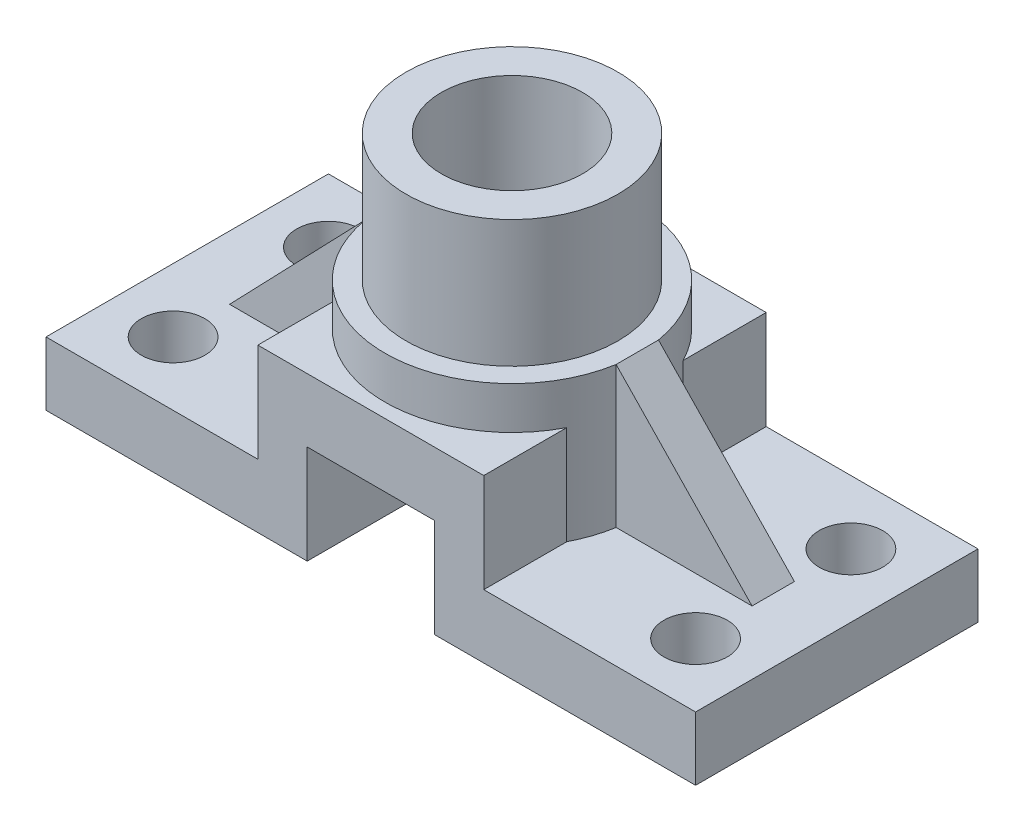
ISO-10303-21;
HEADER;
FILE_DESCRIPTION(('STEP AP214'),'2;1');
FILE_NAME('part.step','',(''),(''),'','','');
FILE_SCHEMA(('AUTOMOTIVE_DESIGN { 1 0 10303 214 1 1 1 1 }'));
ENDSEC;
DATA;
#1=APPLICATION_CONTEXT('core data for automotive mechanical design processes');
#2=APPLICATION_PROTOCOL_DEFINITION('international standard','automotive_design',2000,#1);
#3=PRODUCT_CONTEXT('',#1,'mechanical');
#4=PRODUCT('Part','Part','',(#3));
#5=PRODUCT_RELATED_PRODUCT_CATEGORY('part','',(#4));
#6=PRODUCT_DEFINITION_FORMATION('','',#4);
#7=PRODUCT_DEFINITION_CONTEXT('part definition',#1,'design');
#8=PRODUCT_DEFINITION('design','',#6,#7);
#9=PRODUCT_DEFINITION_SHAPE('','',#8);
#10=(LENGTH_UNIT() NAMED_UNIT(*) SI_UNIT(.MILLI.,.METRE.));
#11=(NAMED_UNIT(*) PLANE_ANGLE_UNIT() SI_UNIT($,.RADIAN.));
#12=(NAMED_UNIT(*) SI_UNIT($,.STERADIAN.) SOLID_ANGLE_UNIT());
#13=UNCERTAINTY_MEASURE_WITH_UNIT(LENGTH_MEASURE(1.E-05),#10,'distance_accuracy_value','');
#14=(GEOMETRIC_REPRESENTATION_CONTEXT(3) GLOBAL_UNCERTAINTY_ASSIGNED_CONTEXT((#13)) GLOBAL_UNIT_ASSIGNED_CONTEXT((#10,
#11,#12)) REPRESENTATION_CONTEXT('',''));
#15=CARTESIAN_POINT('',(0.,0.,0.));
#16=DIRECTION('',(0.,0.,1.));
#17=DIRECTION('',(1.,0.,0.));
#18=AXIS2_PLACEMENT_3D('',#15,#16,#17);
#19=CARTESIAN_POINT('',(-16.,9.,20.));
#20=DIRECTION('',(0.,-1.,0.));
#21=DIRECTION('',(1.,0.,0.));
#22=AXIS2_PLACEMENT_3D('',#19,#20,#21);
#23=PLANE('',#22);
#24=CARTESIAN_POINT('',(-37.,9.,-11.));
#25=DIRECTION('',(0.,-1.,0.));
#26=DIRECTION('',(1.,0.,0.));
#27=AXIS2_PLACEMENT_3D('',#24,#25,#26);
#28=CIRCLE('',#27,4.5);
#29=CARTESIAN_POINT('',(-32.5,9.,-11.));
#30=VERTEX_POINT('',#29);
#31=EDGE_CURVE('E214',#30,#30,#28,.T.);
#32=ORIENTED_EDGE('',*,*,#31,.T.);
#33=EDGE_LOOP('',(#32));
#34=FACE_BOUND('',#33,.T.);
#35=DIRECTION('',(0.,0.,-1.));
#36=VECTOR('',#35,1.);
#37=CARTESIAN_POINT('',(-37.,9.00000000000001,-3.));
#38=LINE('',#37,#36);
#39=CARTESIAN_POINT('',(-37.,9.00000000000001,3.00000000000001));
#40=VERTEX_POINT('',#39);
#41=CARTESIAN_POINT('',(-37.,9.00000000000001,-3.));
#42=VERTEX_POINT('',#41);
#43=EDGE_CURVE('E187',#40,#42,#38,.T.);
#44=ORIENTED_EDGE('',*,*,#43,.T.);
#45=DIRECTION('',(1.,0.,0.));
#46=VECTOR('',#45,1.);
#47=CARTESIAN_POINT('',(-37.,9.00000000000001,-3.));
#48=LINE('',#47,#46);
#49=CARTESIAN_POINT('',(-17.7482393492988,9.00000000000001,-3.));
#50=VERTEX_POINT('',#49);
#51=EDGE_CURVE('E199',#42,#50,#48,.T.);
#52=ORIENTED_EDGE('',*,*,#51,.T.);
#53=CARTESIAN_POINT('',(0.,9.00000000000001,0.));
#54=DIRECTION('',(0.,-1.,0.));
#55=DIRECTION('',(1.,0.,0.));
#56=AXIS2_PLACEMENT_3D('',#53,#54,#55);
#57=CIRCLE('',#56,18.);
#58=CARTESIAN_POINT('',(-16.,9.,-8.24621125123532));
#59=VERTEX_POINT('',#58);
#60=EDGE_CURVE('E276',#59,#50,#57,.F.);
#61=ORIENTED_EDGE('',*,*,#60,.F.);
#62=DIRECTION('',(0.,0.,-1.));
#63=VECTOR('',#62,1.);
#64=CARTESIAN_POINT('',(-16.,9.,20.));
#65=LINE('',#64,#63);
#66=CARTESIAN_POINT('',(-16.,9.,-20.));
#67=VERTEX_POINT('',#66);
#68=EDGE_CURVE('E359',#59,#67,#65,.T.);
#69=ORIENTED_EDGE('',*,*,#68,.T.);
#70=DIRECTION('',(-1.,0.,0.));
#71=VECTOR('',#70,1.);
#72=CARTESIAN_POINT('',(-16.,9.,-20.));
#73=LINE('',#72,#71);
#74=CARTESIAN_POINT('',(-46.,9.,-20.));
#75=VERTEX_POINT('',#74);
#76=EDGE_CURVE('E307',#67,#75,#73,.T.);
#77=ORIENTED_EDGE('',*,*,#76,.T.);
#78=DIRECTION('',(0.,0.,-1.));
#79=VECTOR('',#78,1.);
#80=CARTESIAN_POINT('',(-46.,9.,20.));
#81=LINE('',#80,#79);
#82=CARTESIAN_POINT('',(-46.,9.,20.));
#83=VERTEX_POINT('',#82);
#84=EDGE_CURVE('E328',#83,#75,#81,.T.);
#85=ORIENTED_EDGE('',*,*,#84,.F.);
#86=DIRECTION('',(-1.,0.,0.));
#87=VECTOR('',#86,1.);
#88=CARTESIAN_POINT('',(-16.,9.,20.));
#89=LINE('',#88,#87);
#90=CARTESIAN_POINT('',(-16.,9.,20.));
#91=VERTEX_POINT('',#90);
#92=EDGE_CURVE('E330',#91,#83,#89,.T.);
#93=ORIENTED_EDGE('',*,*,#92,.F.);
#94=CARTESIAN_POINT('',(-16.,9.00000000000001,8.24621125123532));
#95=VERTEX_POINT('',#94);
#96=EDGE_CURVE('E356',#91,#95,#65,.T.);
#97=ORIENTED_EDGE('',*,*,#96,.T.);
#98=CARTESIAN_POINT('',(-17.7482393492988,9.00000000000001,3.));
#99=VERTEX_POINT('',#98);
#100=EDGE_CURVE('E212',#99,#95,#57,.F.);
#101=ORIENTED_EDGE('',*,*,#100,.F.);
#102=DIRECTION('',(-1.,0.,0.));
#103=VECTOR('',#102,1.);
#104=CARTESIAN_POINT('',(-37.,9.00000000000001,3.));
#105=LINE('',#104,#103);
#106=EDGE_CURVE('E206',#99,#40,#105,.T.);
#107=ORIENTED_EDGE('',*,*,#106,.T.);
#108=EDGE_LOOP('',(#44,#52,#61,#69,#77,#85,#93,#97,#101,#107));
#109=FACE_BOUND('',#108,.T.);
#110=CARTESIAN_POINT('',(-37.,9.,11.));
#111=DIRECTION('',(0.,-1.,0.));
#112=DIRECTION('',(1.,0.,0.));
#113=AXIS2_PLACEMENT_3D('',#110,#111,#112);
#114=CIRCLE('',#113,4.5);
#115=CARTESIAN_POINT('',(-32.5,9.,11.));
#116=VERTEX_POINT('',#115);
#117=EDGE_CURVE('E235',#116,#116,#114,.T.);
#118=ORIENTED_EDGE('',*,*,#117,.T.);
#119=EDGE_LOOP('',(#118));
#120=FACE_BOUND('',#119,.T.);
#121=ADVANCED_FACE('F39',(#34,#109,#120),#23,.F.);
#122=CARTESIAN_POINT('',(0.,29.,0.));
#123=DIRECTION('',(0.,-1.,0.));
#124=DIRECTION('',(1.,0.,0.));
#125=AXIS2_PLACEMENT_3D('',#122,#123,#124);
#126=CYLINDRICAL_SURFACE('',#125,18.);
#127=DIRECTION('',(0.,1.,0.));
#128=VECTOR('',#127,1.);
#129=CARTESIAN_POINT('',(-17.7482393492988,-11.1650759520485,-3.));
#130=LINE('',#129,#128);
#131=CARTESIAN_POINT('',(-17.7482393492988,29.,-3.));
#132=VERTEX_POINT('',#131);
#133=EDGE_CURVE('E221',#50,#132,#130,.T.);
#134=ORIENTED_EDGE('',*,*,#133,.T.);
#135=CARTESIAN_POINT('',(0.,29.,0.));
#136=DIRECTION('',(0.,1.,0.));
#137=DIRECTION('',(-1.,0.,0.));
#138=AXIS2_PLACEMENT_3D('',#135,#136,#137);
#139=CIRCLE('',#138,18.);
#140=CARTESIAN_POINT('',(17.7482393492988,29.,-3.));
#141=VERTEX_POINT('',#140);
#142=EDGE_CURVE('E278',#141,#132,#139,.T.);
#143=ORIENTED_EDGE('',*,*,#142,.F.);
#144=DIRECTION('',(0.,1.,0.));
#145=VECTOR('',#144,1.);
#146=CARTESIAN_POINT('',(17.7482393492988,-11.1650759520485,-3.));
#147=LINE('',#146,#145);
#148=CARTESIAN_POINT('',(17.7482393492988,9.,-3.));
#149=VERTEX_POINT('',#148);
#150=EDGE_CURVE('E241',#149,#141,#147,.T.);
#151=ORIENTED_EDGE('',*,*,#150,.F.);
#152=CARTESIAN_POINT('',(0.,9.00000000000001,0.));
#153=DIRECTION('',(0.,1.,0.));
#154=DIRECTION('',(-1.,0.,0.));
#155=AXIS2_PLACEMENT_3D('',#152,#153,#154);
#156=CIRCLE('',#155,18.);
#157=CARTESIAN_POINT('',(16.,9.,-8.24621125123532));
#158=VERTEX_POINT('',#157);
#159=EDGE_CURVE('E63',#149,#158,#156,.T.);
#160=ORIENTED_EDGE('',*,*,#159,.T.);
#161=DIRECTION('',(0.,-1.,0.));
#162=VECTOR('',#161,1.);
#163=CARTESIAN_POINT('',(16.,29.,-8.24621125123533));
#164=LINE('',#163,#162);
#165=CARTESIAN_POINT('',(16.,23.,-8.24621125123533));
#166=VERTEX_POINT('',#165);
#167=EDGE_CURVE('E291',#158,#166,#164,.F.);
#168=ORIENTED_EDGE('',*,*,#167,.T.);
#169=CARTESIAN_POINT('',(0.,23.,0.));
#170=DIRECTION('',(0.,-1.,0.));
#171=DIRECTION('',(0.,0.,-1.));
#172=AXIS2_PLACEMENT_3D('',#169,#170,#171);
#173=CIRCLE('',#172,18.);
#174=CARTESIAN_POINT('',(-16.,23.,-8.24621125123531));
#175=VERTEX_POINT('',#174);
#176=EDGE_CURVE('E286',#166,#175,#173,.F.);
#177=ORIENTED_EDGE('',*,*,#176,.T.);
#178=DIRECTION('',(0.,-1.,0.));
#179=VECTOR('',#178,1.);
#180=CARTESIAN_POINT('',(-16.,29.,-8.24621125123531));
#181=LINE('',#180,#179);
#182=EDGE_CURVE('E281',#175,#59,#181,.T.);
#183=ORIENTED_EDGE('',*,*,#182,.T.);
#184=ORIENTED_EDGE('',*,*,#60,.T.);
#185=EDGE_LOOP('',(#134,#143,#151,#160,#168,#177,#183,#184));
#186=FACE_BOUND('',#185,.T.);
#187=ADVANCED_FACE('F420',(#186),#126,.T.);
#188=DIRECTION('',(0.,1.,0.));
#189=VECTOR('',#188,1.);
#190=CARTESIAN_POINT('',(-17.7482393492988,-11.1650759520485,3.));
#191=LINE('',#190,#189);
#192=CARTESIAN_POINT('',(-17.7482393492988,29.,3.00000000000001));
#193=VERTEX_POINT('',#192);
#194=EDGE_CURVE('E203',#99,#193,#191,.T.);
#195=ORIENTED_EDGE('',*,*,#194,.F.);
#196=ORIENTED_EDGE('',*,*,#100,.T.);
#197=DIRECTION('',(0.,-1.,0.));
#198=VECTOR('',#197,1.);
#199=CARTESIAN_POINT('',(-16.,29.,8.24621125123531));
#200=LINE('',#199,#198);
#201=CARTESIAN_POINT('',(-16.,23.,8.24621125123531));
#202=VERTEX_POINT('',#201);
#203=EDGE_CURVE('E298',#95,#202,#200,.F.);
#204=ORIENTED_EDGE('',*,*,#203,.T.);
#205=CARTESIAN_POINT('',(16.,23.,8.24621125123533));
#206=VERTEX_POINT('',#205);
#207=EDGE_CURVE('E294',#202,#206,#173,.F.);
#208=ORIENTED_EDGE('',*,*,#207,.T.);
#209=DIRECTION('',(0.,-1.,0.));
#210=VECTOR('',#209,1.);
#211=CARTESIAN_POINT('',(16.,29.,8.24621125123533));
#212=LINE('',#211,#210);
#213=CARTESIAN_POINT('',(16.,9.,8.24621125123532));
#214=VERTEX_POINT('',#213);
#215=EDGE_CURVE('E297',#206,#214,#212,.T.);
#216=ORIENTED_EDGE('',*,*,#215,.T.);
#217=CARTESIAN_POINT('',(17.7482393492988,9.00000000000001,3.));
#218=VERTEX_POINT('',#217);
#219=EDGE_CURVE('E284',#214,#218,#156,.T.);
#220=ORIENTED_EDGE('',*,*,#219,.T.);
#221=DIRECTION('',(0.,1.,0.));
#222=VECTOR('',#221,1.);
#223=CARTESIAN_POINT('',(17.7482393492988,-11.1650759520485,3.));
#224=LINE('',#223,#222);
#225=CARTESIAN_POINT('',(17.7482393492988,29.,3.00000000000001));
#226=VERTEX_POINT('',#225);
#227=EDGE_CURVE('E243',#218,#226,#224,.T.);
#228=ORIENTED_EDGE('',*,*,#227,.T.);
#229=EDGE_CURVE('E282',#193,#226,#139,.T.);
#230=ORIENTED_EDGE('',*,*,#229,.F.);
#231=EDGE_LOOP('',(#195,#196,#204,#208,#216,#220,#228,#230));
#232=FACE_BOUND('',#231,.T.);
#233=ADVANCED_FACE('F426',(#232),#126,.T.);
#234=CARTESIAN_POINT('',(-9.,0.,20.));
#235=DIRECTION('',(-1.,0.,0.));
#236=DIRECTION('',(0.,0.,1.));
#237=AXIS2_PLACEMENT_3D('',#234,#235,#236);
#238=PLANE('',#237);
#239=DIRECTION('',(0.,0.,-1.));
#240=VECTOR('',#239,1.);
#241=CARTESIAN_POINT('',(-9.,14.,20.));
#242=LINE('',#241,#240);
#243=CARTESIAN_POINT('',(-9.,14.,20.));
#244=VERTEX_POINT('',#243);
#245=CARTESIAN_POINT('',(-9.,14.,-20.));
#246=VERTEX_POINT('',#245);
#247=EDGE_CURVE('E384',#244,#246,#242,.T.);
#248=ORIENTED_EDGE('',*,*,#247,.F.);
#249=DIRECTION('',(0.,1.,0.));
#250=VECTOR('',#249,1.);
#251=CARTESIAN_POINT('',(-9.,0.,20.));
#252=LINE('',#251,#250);
#253=CARTESIAN_POINT('',(-9.,0.,20.));
#254=VERTEX_POINT('',#253);
#255=EDGE_CURVE('E310',#254,#244,#252,.T.);
#256=ORIENTED_EDGE('',*,*,#255,.F.);
#257=DIRECTION('',(0.,0.,-1.));
#258=VECTOR('',#257,1.);
#259=CARTESIAN_POINT('',(-9.,0.,20.));
#260=LINE('',#259,#258);
#261=CARTESIAN_POINT('',(-9.,0.,-20.));
#262=VERTEX_POINT('',#261);
#263=EDGE_CURVE('E389',#254,#262,#260,.T.);
#264=ORIENTED_EDGE('',*,*,#263,.T.);
#265=DIRECTION('',(0.,1.,0.));
#266=VECTOR('',#265,1.);
#267=CARTESIAN_POINT('',(-9.,0.,-20.));
#268=LINE('',#267,#266);
#269=EDGE_CURVE('E331',#262,#246,#268,.T.);
#270=ORIENTED_EDGE('',*,*,#269,.T.);
#271=EDGE_LOOP('',(#248,#256,#264,#270));
#272=FACE_BOUND('',#271,.T.);
#273=ADVANCED_FACE('F465',(#272),#238,.F.);
#274=CARTESIAN_POINT('',(9.,14.,20.));
#275=DIRECTION('',(1.,0.,0.));
#276=DIRECTION('',(0.,0.,-1.));
#277=AXIS2_PLACEMENT_3D('',#274,#275,#276);
#278=PLANE('',#277);
#279=DIRECTION('',(0.,-1.,0.));
#280=VECTOR('',#279,1.);
#281=CARTESIAN_POINT('',(9.,14.,-20.));
#282=LINE('',#281,#280);
#283=CARTESIAN_POINT('',(9.,14.,-20.));
#284=VERTEX_POINT('',#283);
#285=CARTESIAN_POINT('',(9.,0.,-20.));
#286=VERTEX_POINT('',#285);
#287=EDGE_CURVE('E337',#284,#286,#282,.T.);
#288=ORIENTED_EDGE('',*,*,#287,.T.);
#289=DIRECTION('',(0.,0.,-1.));
#290=VECTOR('',#289,1.);
#291=CARTESIAN_POINT('',(9.,0.,20.));
#292=LINE('',#291,#290);
#293=CARTESIAN_POINT('',(9.,0.,20.));
#294=VERTEX_POINT('',#293);
#295=EDGE_CURVE('E379',#294,#286,#292,.T.);
#296=ORIENTED_EDGE('',*,*,#295,.F.);
#297=DIRECTION('',(0.,-1.,0.));
#298=VECTOR('',#297,1.);
#299=CARTESIAN_POINT('',(9.,14.,20.));
#300=LINE('',#299,#298);
#301=CARTESIAN_POINT('',(9.,14.,20.));
#302=VERTEX_POINT('',#301);
#303=EDGE_CURVE('E311',#302,#294,#300,.T.);
#304=ORIENTED_EDGE('',*,*,#303,.F.);
#305=DIRECTION('',(0.,0.,-1.));
#306=VECTOR('',#305,1.);
#307=CARTESIAN_POINT('',(9.,14.,20.));
#308=LINE('',#307,#306);
#309=EDGE_CURVE('E382',#302,#284,#308,.T.);
#310=ORIENTED_EDGE('',*,*,#309,.T.);
#311=EDGE_LOOP('',(#288,#296,#304,#310));
#312=FACE_BOUND('',#311,.T.);
#313=ADVANCED_FACE('F446',(#312),#278,.F.);
#314=CARTESIAN_POINT('',(16.,9.,20.));
#315=DIRECTION('',(-1.,0.,0.));
#316=DIRECTION('',(0.,0.,1.));
#317=AXIS2_PLACEMENT_3D('',#314,#315,#316);
#318=PLANE('',#317);
#319=ORIENTED_EDGE('',*,*,#167,.F.);
#320=DIRECTION('',(0.,0.,-1.));
#321=VECTOR('',#320,1.);
#322=CARTESIAN_POINT('',(16.,9.,20.));
#323=LINE('',#322,#321);
#324=CARTESIAN_POINT('',(16.,9.,-20.));
#325=VERTEX_POINT('',#324);
#326=EDGE_CURVE('E367',#158,#325,#323,.T.);
#327=ORIENTED_EDGE('',*,*,#326,.T.);
#328=DIRECTION('',(0.,1.,0.));
#329=VECTOR('',#328,1.);
#330=CARTESIAN_POINT('',(16.,9.,-20.));
#331=LINE('',#330,#329);
#332=CARTESIAN_POINT('',(16.,23.,-20.));
#333=VERTEX_POINT('',#332);
#334=EDGE_CURVE('E350',#325,#333,#331,.T.);
#335=ORIENTED_EDGE('',*,*,#334,.T.);
#336=DIRECTION('',(0.,0.,-1.));
#337=VECTOR('',#336,1.);
#338=CARTESIAN_POINT('',(16.,23.,20.));
#339=LINE('',#338,#337);
#340=EDGE_CURVE('E368',#166,#333,#339,.T.);
#341=ORIENTED_EDGE('',*,*,#340,.F.);
#342=EDGE_LOOP('',(#319,#327,#335,#341));
#343=FACE_BOUND('',#342,.T.);
#344=ADVANCED_FACE('F441',(#343),#318,.F.);
#345=ORIENTED_EDGE('',*,*,#215,.F.);
#346=CARTESIAN_POINT('',(16.,23.,20.));
#347=VERTEX_POINT('',#346);
#348=EDGE_CURVE('E370',#347,#206,#339,.T.);
#349=ORIENTED_EDGE('',*,*,#348,.F.);
#350=DIRECTION('',(0.,1.,0.));
#351=VECTOR('',#350,1.);
#352=CARTESIAN_POINT('',(16.,9.,20.));
#353=LINE('',#352,#351);
#354=CARTESIAN_POINT('',(16.,9.,20.));
#355=VERTEX_POINT('',#354);
#356=EDGE_CURVE('E321',#355,#347,#353,.T.);
#357=ORIENTED_EDGE('',*,*,#356,.F.);
#358=EDGE_CURVE('E371',#355,#214,#323,.T.);
#359=ORIENTED_EDGE('',*,*,#358,.T.);
#360=EDGE_LOOP('',(#345,#349,#357,#359));
#361=FACE_BOUND('',#360,.T.);
#362=ADVANCED_FACE('F450',(#361),#318,.F.);
#363=CARTESIAN_POINT('',(16.,23.,20.));
#364=DIRECTION('',(0.,-1.,0.));
#365=DIRECTION('',(0.,0.,-1.));
#366=AXIS2_PLACEMENT_3D('',#363,#364,#365);
#367=PLANE('',#366);
#368=ORIENTED_EDGE('',*,*,#207,.F.);
#369=DIRECTION('',(0.,0.,-1.));
#370=VECTOR('',#369,1.);
#371=CARTESIAN_POINT('',(-16.,23.,20.));
#372=LINE('',#371,#370);
#373=CARTESIAN_POINT('',(-16.,23.,20.));
#374=VERTEX_POINT('',#373);
#375=EDGE_CURVE('E361',#374,#202,#372,.T.);
#376=ORIENTED_EDGE('',*,*,#375,.F.);
#377=DIRECTION('',(-1.,0.,0.));
#378=VECTOR('',#377,1.);
#379=CARTESIAN_POINT('',(16.,23.,20.));
#380=LINE('',#379,#378);
#381=EDGE_CURVE('E323',#347,#374,#380,.T.);
#382=ORIENTED_EDGE('',*,*,#381,.F.);
#383=ORIENTED_EDGE('',*,*,#348,.T.);
#384=EDGE_LOOP('',(#368,#376,#382,#383));
#385=FACE_BOUND('',#384,.T.);
#386=ADVANCED_FACE('F436',(#385),#367,.F.);
#387=CARTESIAN_POINT('',(-16.,23.,20.));
#388=DIRECTION('',(1.,0.,0.));
#389=DIRECTION('',(0.,0.,-1.));
#390=AXIS2_PLACEMENT_3D('',#387,#388,#389);
#391=PLANE('',#390);
#392=ORIENTED_EDGE('',*,*,#203,.F.);
#393=ORIENTED_EDGE('',*,*,#96,.F.);
#394=DIRECTION('',(0.,-1.,0.));
#395=VECTOR('',#394,1.);
#396=CARTESIAN_POINT('',(-16.,23.,20.));
#397=LINE('',#396,#395);
#398=EDGE_CURVE('E324',#374,#91,#397,.T.);
#399=ORIENTED_EDGE('',*,*,#398,.F.);
#400=ORIENTED_EDGE('',*,*,#375,.T.);
#401=EDGE_LOOP('',(#392,#393,#399,#400));
#402=FACE_BOUND('',#401,.T.);
#403=ADVANCED_FACE('F435',(#402),#391,.F.);
#404=ORIENTED_EDGE('',*,*,#182,.F.);
#405=CARTESIAN_POINT('',(-16.,23.,-20.));
#406=VERTEX_POINT('',#405);
#407=EDGE_CURVE('E362',#175,#406,#372,.T.);
#408=ORIENTED_EDGE('',*,*,#407,.T.);
#409=DIRECTION('',(0.,-1.,0.));
#410=VECTOR('',#409,1.);
#411=CARTESIAN_POINT('',(-16.,23.,-20.));
#412=LINE('',#411,#410);
#413=EDGE_CURVE('E351',#406,#67,#412,.T.);
#414=ORIENTED_EDGE('',*,*,#413,.T.);
#415=ORIENTED_EDGE('',*,*,#68,.F.);
#416=EDGE_LOOP('',(#404,#408,#414,#415));
#417=FACE_BOUND('',#416,.T.);
#418=ADVANCED_FACE('F434',(#417),#391,.F.);
#419=CARTESIAN_POINT('',(-46.,9.,20.));
#420=DIRECTION('',(1.,0.,0.));
#421=DIRECTION('',(0.,0.,-1.));
#422=AXIS2_PLACEMENT_3D('',#419,#420,#421);
#423=PLANE('',#422);
#424=DIRECTION('',(0.,-1.,0.));
#425=VECTOR('',#424,1.);
#426=CARTESIAN_POINT('',(-46.,9.,-20.));
#427=LINE('',#426,#425);
#428=CARTESIAN_POINT('',(-46.,0.,-20.));
#429=VERTEX_POINT('',#428);
#430=EDGE_CURVE('E305',#75,#429,#427,.T.);
#431=ORIENTED_EDGE('',*,*,#430,.T.);
#432=DIRECTION('',(0.,0.,-1.));
#433=VECTOR('',#432,1.);
#434=CARTESIAN_POINT('',(-46.,0.,20.));
#435=LINE('',#434,#433);
#436=CARTESIAN_POINT('',(-46.,0.,20.));
#437=VERTEX_POINT('',#436);
#438=EDGE_CURVE('E393',#437,#429,#435,.T.);
#439=ORIENTED_EDGE('',*,*,#438,.F.);
#440=DIRECTION('',(0.,-1.,0.));
#441=VECTOR('',#440,1.);
#442=CARTESIAN_POINT('',(-46.,9.,20.));
#443=LINE('',#442,#441);
#444=EDGE_CURVE('E303',#83,#437,#443,.T.);
#445=ORIENTED_EDGE('',*,*,#444,.F.);
#446=ORIENTED_EDGE('',*,*,#84,.T.);
#447=EDGE_LOOP('',(#431,#439,#445,#446));
#448=FACE_BOUND('',#447,.T.);
#449=ADVANCED_FACE('F41',(#448),#423,.F.);
#450=CARTESIAN_POINT('',(-46.,0.,20.));
#451=DIRECTION('',(0.,1.,0.));
#452=DIRECTION('',(0.,0.,1.));
#453=AXIS2_PLACEMENT_3D('',#450,#451,#452);
#454=PLANE('',#453);
#455=CARTESIAN_POINT('',(-37.,0.,11.));
#456=DIRECTION('',(0.,-1.,0.));
#457=DIRECTION('',(1.,0.,0.));
#458=AXIS2_PLACEMENT_3D('',#455,#456,#457);
#459=CIRCLE('',#458,4.5);
#460=CARTESIAN_POINT('',(-32.5,0.,11.));
#461=VERTEX_POINT('',#460);
#462=EDGE_CURVE('E226',#461,#461,#459,.T.);
#463=ORIENTED_EDGE('',*,*,#462,.F.);
#464=EDGE_LOOP('',(#463));
#465=FACE_BOUND('',#464,.T.);
#466=CARTESIAN_POINT('',(-37.,0.,-11.));
#467=DIRECTION('',(0.,-1.,0.));
#468=DIRECTION('',(1.,0.,0.));
#469=AXIS2_PLACEMENT_3D('',#466,#467,#468);
#470=CIRCLE('',#469,4.5);
#471=CARTESIAN_POINT('',(-32.5,0.,-11.));
#472=VERTEX_POINT('',#471);
#473=EDGE_CURVE('E217',#472,#472,#470,.T.);
#474=ORIENTED_EDGE('',*,*,#473,.F.);
#475=EDGE_LOOP('',(#474));
#476=FACE_BOUND('',#475,.T.);
#477=DIRECTION('',(1.,0.,0.));
#478=VECTOR('',#477,1.);
#479=CARTESIAN_POINT('',(-46.,0.,-20.));
#480=LINE('',#479,#478);
#481=EDGE_CURVE('E335',#429,#262,#480,.T.);
#482=ORIENTED_EDGE('',*,*,#481,.T.);
#483=ORIENTED_EDGE('',*,*,#263,.F.);
#484=DIRECTION('',(1.,0.,0.));
#485=VECTOR('',#484,1.);
#486=CARTESIAN_POINT('',(-46.,0.,20.));
#487=LINE('',#486,#485);
#488=EDGE_CURVE('E308',#437,#254,#487,.T.);
#489=ORIENTED_EDGE('',*,*,#488,.F.);
#490=ORIENTED_EDGE('',*,*,#438,.T.);
#491=EDGE_LOOP('',(#482,#483,#489,#490));
#492=FACE_BOUND('',#491,.T.);
#493=ADVANCED_FACE('F467',(#465,#476,#492),#454,.F.);
#494=CARTESIAN_POINT('',(-9.,14.,20.));
#495=DIRECTION('',(0.,1.,0.));
#496=DIRECTION('',(0.,0.,1.));
#497=AXIS2_PLACEMENT_3D('',#494,#495,#496);
#498=PLANE('',#497);
#499=CARTESIAN_POINT('',(0.,14.,0.));
#500=DIRECTION('',(0.,1.,0.));
#501=DIRECTION('',(0.,0.,1.));
#502=AXIS2_PLACEMENT_3D('',#499,#500,#501);
#503=CIRCLE('',#502,7.);
#504=CARTESIAN_POINT('',(0.,14.,7.));
#505=VERTEX_POINT('',#504);
#506=EDGE_CURVE('E270',#505,#505,#503,.T.);
#507=ORIENTED_EDGE('',*,*,#506,.T.);
#508=EDGE_LOOP('',(#507));
#509=FACE_BOUND('',#508,.T.);
#510=ORIENTED_EDGE('',*,*,#247,.T.);
#511=DIRECTION('',(1.,0.,0.));
#512=VECTOR('',#511,1.);
#513=CARTESIAN_POINT('',(-9.,14.,-20.));
#514=LINE('',#513,#512);
#515=EDGE_CURVE('E338',#246,#284,#514,.T.);
#516=ORIENTED_EDGE('',*,*,#515,.T.);
#517=ORIENTED_EDGE('',*,*,#309,.F.);
#518=DIRECTION('',(1.,0.,0.));
#519=VECTOR('',#518,1.);
#520=CARTESIAN_POINT('',(-9.,14.,20.));
#521=LINE('',#520,#519);
#522=EDGE_CURVE('E313',#244,#302,#521,.T.);
#523=ORIENTED_EDGE('',*,*,#522,.F.);
#524=EDGE_LOOP('',(#510,#516,#517,#523));
#525=FACE_BOUND('',#524,.T.);
#526=ADVANCED_FACE('F398',(#509,#525),#498,.F.);
#527=CARTESIAN_POINT('',(9.,0.,20.));
#528=DIRECTION('',(0.,1.,0.));
#529=DIRECTION('',(0.,0.,1.));
#530=AXIS2_PLACEMENT_3D('',#527,#528,#529);
#531=PLANE('',#530);
#532=CARTESIAN_POINT('',(37.,0.,11.));
#533=DIRECTION('',(0.,1.,0.));
#534=DIRECTION('',(-1.,0.,0.));
#535=AXIS2_PLACEMENT_3D('',#532,#533,#534);
#536=CIRCLE('',#535,4.5);
#537=CARTESIAN_POINT('',(32.5,0.,11.));
#538=VERTEX_POINT('',#537);
#539=EDGE_CURVE('E251',#538,#538,#536,.T.);
#540=ORIENTED_EDGE('',*,*,#539,.T.);
#541=EDGE_LOOP('',(#540));
#542=FACE_BOUND('',#541,.T.);
#543=CARTESIAN_POINT('',(37.,0.,-11.));
#544=DIRECTION('',(0.,1.,0.));
#545=DIRECTION('',(-1.,0.,0.));
#546=AXIS2_PLACEMENT_3D('',#543,#544,#545);
#547=CIRCLE('',#546,4.5);
#548=CARTESIAN_POINT('',(32.5,0.,-11.));
#549=VERTEX_POINT('',#548);
#550=EDGE_CURVE('E257',#549,#549,#547,.T.);
#551=ORIENTED_EDGE('',*,*,#550,.T.);
#552=EDGE_LOOP('',(#551));
#553=FACE_BOUND('',#552,.T.);
#554=DIRECTION('',(1.,0.,0.));
#555=VECTOR('',#554,1.);
#556=CARTESIAN_POINT('',(9.,0.,-20.));
#557=LINE('',#556,#555);
#558=CARTESIAN_POINT('',(46.,0.,-20.));
#559=VERTEX_POINT('',#558);
#560=EDGE_CURVE('E342',#286,#559,#557,.T.);
#561=ORIENTED_EDGE('',*,*,#560,.T.);
#562=DIRECTION('',(0.,0.,-1.));
#563=VECTOR('',#562,1.);
#564=CARTESIAN_POINT('',(46.,0.,20.));
#565=LINE('',#564,#563);
#566=CARTESIAN_POINT('',(46.,0.,20.));
#567=VERTEX_POINT('',#566);
#568=EDGE_CURVE('E380',#567,#559,#565,.T.);
#569=ORIENTED_EDGE('',*,*,#568,.F.);
#570=DIRECTION('',(1.,0.,0.));
#571=VECTOR('',#570,1.);
#572=CARTESIAN_POINT('',(9.,0.,20.));
#573=LINE('',#572,#571);
#574=EDGE_CURVE('E312',#294,#567,#573,.T.);
#575=ORIENTED_EDGE('',*,*,#574,.F.);
#576=ORIENTED_EDGE('',*,*,#295,.T.);
#577=EDGE_LOOP('',(#561,#569,#575,#576));
#578=FACE_BOUND('',#577,.T.);
#579=ADVANCED_FACE('F457',(#542,#553,#578),#531,.F.);
#580=CARTESIAN_POINT('',(46.,0.,20.));
#581=DIRECTION('',(-1.,0.,0.));
#582=DIRECTION('',(0.,0.,1.));
#583=AXIS2_PLACEMENT_3D('',#580,#581,#582);
#584=PLANE('',#583);
#585=DIRECTION('',(0.,1.,0.));
#586=VECTOR('',#585,1.);
#587=CARTESIAN_POINT('',(46.,0.,-20.));
#588=LINE('',#587,#586);
#589=CARTESIAN_POINT('',(46.,9.,-20.));
#590=VERTEX_POINT('',#589);
#591=EDGE_CURVE('E343',#559,#590,#588,.T.);
#592=ORIENTED_EDGE('',*,*,#591,.T.);
#593=DIRECTION('',(0.,0.,-1.));
#594=VECTOR('',#593,1.);
#595=CARTESIAN_POINT('',(46.,9.,20.));
#596=LINE('',#595,#594);
#597=CARTESIAN_POINT('',(46.,9.,20.));
#598=VERTEX_POINT('',#597);
#599=EDGE_CURVE('E372',#598,#590,#596,.T.);
#600=ORIENTED_EDGE('',*,*,#599,.F.);
#601=DIRECTION('',(0.,1.,0.));
#602=VECTOR('',#601,1.);
#603=CARTESIAN_POINT('',(46.,0.,20.));
#604=LINE('',#603,#602);
#605=EDGE_CURVE('E320',#567,#598,#604,.T.);
#606=ORIENTED_EDGE('',*,*,#605,.F.);
#607=ORIENTED_EDGE('',*,*,#568,.T.);
#608=EDGE_LOOP('',(#592,#600,#606,#607));
#609=FACE_BOUND('',#608,.T.);
#610=ADVANCED_FACE('F455',(#609),#584,.F.);
#611=CARTESIAN_POINT('',(46.,9.,20.));
#612=DIRECTION('',(0.,-1.,0.));
#613=DIRECTION('',(1.,0.,0.));
#614=AXIS2_PLACEMENT_3D('',#611,#612,#613);
#615=PLANE('',#614);
#616=CARTESIAN_POINT('',(37.,9.,-11.));
#617=DIRECTION('',(0.,1.,0.));
#618=DIRECTION('',(-1.,0.,0.));
#619=AXIS2_PLACEMENT_3D('',#616,#617,#618);
#620=CIRCLE('',#619,4.5);
#621=CARTESIAN_POINT('',(32.5,9.,-11.));
#622=VERTEX_POINT('',#621);
#623=EDGE_CURVE('E252',#622,#622,#620,.T.);
#624=ORIENTED_EDGE('',*,*,#623,.F.);
#625=EDGE_LOOP('',(#624));
#626=FACE_BOUND('',#625,.T.);
#627=DIRECTION('',(-1.,0.,0.));
#628=VECTOR('',#627,1.);
#629=CARTESIAN_POINT('',(37.,9.,-3.));
#630=LINE('',#629,#628);
#631=CARTESIAN_POINT('',(37.,9.,-3.));
#632=VERTEX_POINT('',#631);
#633=EDGE_CURVE('E53',#632,#149,#630,.T.);
#634=ORIENTED_EDGE('',*,*,#633,.F.);
#635=DIRECTION('',(0.,0.,-1.));
#636=VECTOR('',#635,1.);
#637=CARTESIAN_POINT('',(37.,9.,-3.));
#638=LINE('',#637,#636);
#639=CARTESIAN_POINT('',(37.,9.,3.00000000000001));
#640=VERTEX_POINT('',#639);
#641=EDGE_CURVE('E242',#640,#632,#638,.T.);
#642=ORIENTED_EDGE('',*,*,#641,.F.);
#643=DIRECTION('',(1.,0.,0.));
#644=VECTOR('',#643,1.);
#645=CARTESIAN_POINT('',(37.,9.,3.));
#646=LINE('',#645,#644);
#647=EDGE_CURVE('E247',#218,#640,#646,.T.);
#648=ORIENTED_EDGE('',*,*,#647,.F.);
#649=ORIENTED_EDGE('',*,*,#219,.F.);
#650=ORIENTED_EDGE('',*,*,#358,.F.);
#651=DIRECTION('',(-1.,0.,0.));
#652=VECTOR('',#651,1.);
#653=CARTESIAN_POINT('',(46.,9.,20.));
#654=LINE('',#653,#652);
#655=EDGE_CURVE('E317',#598,#355,#654,.T.);
#656=ORIENTED_EDGE('',*,*,#655,.F.);
#657=ORIENTED_EDGE('',*,*,#599,.T.);
#658=DIRECTION('',(-1.,0.,0.));
#659=VECTOR('',#658,1.);
#660=CARTESIAN_POINT('',(46.,9.,-20.));
#661=LINE('',#660,#659);
#662=EDGE_CURVE('E341',#590,#325,#661,.T.);
#663=ORIENTED_EDGE('',*,*,#662,.T.);
#664=ORIENTED_EDGE('',*,*,#326,.F.);
#665=ORIENTED_EDGE('',*,*,#159,.F.);
#666=EDGE_LOOP('',(#634,#642,#648,#649,#650,#656,#657,#663,#664,#665));
#667=FACE_BOUND('',#666,.T.);
#668=CARTESIAN_POINT('',(37.,9.,11.));
#669=DIRECTION('',(0.,1.,0.));
#670=DIRECTION('',(-1.,0.,0.));
#671=AXIS2_PLACEMENT_3D('',#668,#669,#670);
#672=CIRCLE('',#671,4.5);
#673=CARTESIAN_POINT('',(32.5,9.,11.));
#674=VERTEX_POINT('',#673);
#675=EDGE_CURVE('E260',#674,#674,#672,.T.);
#676=ORIENTED_EDGE('',*,*,#675,.F.);
#677=EDGE_LOOP('',(#676));
#678=FACE_BOUND('',#677,.T.);
#679=ADVANCED_FACE('F445',(#626,#667,#678),#615,.F.);
#680=ORIENTED_EDGE('',*,*,#176,.F.);
#681=ORIENTED_EDGE('',*,*,#340,.T.);
#682=DIRECTION('',(-1.,0.,0.));
#683=VECTOR('',#682,1.);
#684=CARTESIAN_POINT('',(16.,23.,-20.));
#685=LINE('',#684,#683);
#686=EDGE_CURVE('E348',#333,#406,#685,.T.);
#687=ORIENTED_EDGE('',*,*,#686,.T.);
#688=ORIENTED_EDGE('',*,*,#407,.F.);
#689=EDGE_LOOP('',(#680,#681,#687,#688));
#690=FACE_BOUND('',#689,.T.);
#691=ADVANCED_FACE('F437',(#690),#367,.F.);
#692=CARTESIAN_POINT('',(0.,0.,20.));
#693=DIRECTION('',(0.,0.,1.));
#694=DIRECTION('',(1.,0.,0.));
#695=AXIS2_PLACEMENT_3D('',#692,#693,#694);
#696=PLANE('',#695);
#697=ORIENTED_EDGE('',*,*,#444,.T.);
#698=ORIENTED_EDGE('',*,*,#488,.T.);
#699=ORIENTED_EDGE('',*,*,#255,.T.);
#700=ORIENTED_EDGE('',*,*,#522,.T.);
#701=ORIENTED_EDGE('',*,*,#303,.T.);
#702=ORIENTED_EDGE('',*,*,#574,.T.);
#703=ORIENTED_EDGE('',*,*,#605,.T.);
#704=ORIENTED_EDGE('',*,*,#655,.T.);
#705=ORIENTED_EDGE('',*,*,#356,.T.);
#706=ORIENTED_EDGE('',*,*,#381,.T.);
#707=ORIENTED_EDGE('',*,*,#398,.T.);
#708=ORIENTED_EDGE('',*,*,#92,.T.);
#709=EDGE_LOOP('',(#697,#698,#699,#700,#701,#702,#703,#704,#705,#706,#707,#708));
#710=FACE_BOUND('',#709,.T.);
#711=ADVANCED_FACE('F442',(#710),#696,.T.);
#712=CARTESIAN_POINT('',(0.,0.,-20.));
#713=DIRECTION('',(0.,0.,1.));
#714=DIRECTION('',(1.,0.,0.));
#715=AXIS2_PLACEMENT_3D('',#712,#713,#714);
#716=PLANE('',#715);
#717=ORIENTED_EDGE('',*,*,#430,.F.);
#718=ORIENTED_EDGE('',*,*,#76,.F.);
#719=ORIENTED_EDGE('',*,*,#413,.F.);
#720=ORIENTED_EDGE('',*,*,#686,.F.);
#721=ORIENTED_EDGE('',*,*,#334,.F.);
#722=ORIENTED_EDGE('',*,*,#662,.F.);
#723=ORIENTED_EDGE('',*,*,#591,.F.);
#724=ORIENTED_EDGE('',*,*,#560,.F.);
#725=ORIENTED_EDGE('',*,*,#287,.F.);
#726=ORIENTED_EDGE('',*,*,#515,.F.);
#727=ORIENTED_EDGE('',*,*,#269,.F.);
#728=ORIENTED_EDGE('',*,*,#481,.F.);
#729=EDGE_LOOP('',(#717,#718,#719,#720,#721,#722,#723,#724,#725,#726,#727,#728));
#730=FACE_BOUND('',#729,.T.);
#731=ADVANCED_FACE('F429',(#730),#716,.F.);
#732=CARTESIAN_POINT('',(0.,29.,0.));
#733=DIRECTION('',(0.,1.,0.));
#734=DIRECTION('',(-1.,0.,0.));
#735=AXIS2_PLACEMENT_3D('',#732,#733,#734);
#736=PLANE('',#735);
#737=DIRECTION('',(0.,0.,1.));
#738=VECTOR('',#737,1.);
#739=CARTESIAN_POINT('',(-17.7482393492988,29.,-20.));
#740=LINE('',#739,#738);
#741=EDGE_CURVE('E207',#132,#193,#740,.T.);
#742=ORIENTED_EDGE('',*,*,#741,.T.);
#743=ORIENTED_EDGE('',*,*,#229,.T.);
#744=DIRECTION('',(0.,0.,1.));
#745=VECTOR('',#744,1.);
#746=CARTESIAN_POINT('',(17.7482393492988,29.,-20.));
#747=LINE('',#746,#745);
#748=EDGE_CURVE('E236',#141,#226,#747,.T.);
#749=ORIENTED_EDGE('',*,*,#748,.F.);
#750=ORIENTED_EDGE('',*,*,#142,.T.);
#751=EDGE_LOOP('',(#742,#743,#749,#750));
#752=FACE_BOUND('',#751,.T.);
#753=CARTESIAN_POINT('',(0.,29.,0.));
#754=DIRECTION('',(0.,1.,0.));
#755=DIRECTION('',(-1.,0.,0.));
#756=AXIS2_PLACEMENT_3D('',#753,#754,#755);
#757=CIRCLE('',#756,15.);
#758=CARTESIAN_POINT('',(-15.,29.,0.));
#759=VERTEX_POINT('',#758);
#760=EDGE_CURVE('E50',#759,#759,#757,.T.);
#761=ORIENTED_EDGE('',*,*,#760,.F.);
#762=EDGE_LOOP('',(#761));
#763=FACE_BOUND('',#762,.T.);
#764=ADVANCED_FACE('F531',(#752,#763),#736,.T.);
#765=CARTESIAN_POINT('',(0.,47.,0.));
#766=DIRECTION('',(0.,-1.,0.));
#767=DIRECTION('',(1.,0.,0.));
#768=AXIS2_PLACEMENT_3D('',#765,#766,#767);
#769=CYLINDRICAL_SURFACE('',#768,15.);
#770=CARTESIAN_POINT('',(0.,47.,0.));
#771=DIRECTION('',(0.,1.,0.));
#772=DIRECTION('',(-1.,0.,0.));
#773=AXIS2_PLACEMENT_3D('',#770,#771,#772);
#774=CIRCLE('',#773,15.);
#775=CARTESIAN_POINT('',(-15.,47.,0.));
#776=VERTEX_POINT('',#775);
#777=EDGE_CURVE('E271',#776,#776,#774,.T.);
#778=ORIENTED_EDGE('',*,*,#777,.F.);
#779=EDGE_LOOP('',(#778));
#780=FACE_BOUND('',#779,.T.);
#781=ORIENTED_EDGE('',*,*,#760,.T.);
#782=EDGE_LOOP('',(#781));
#783=FACE_BOUND('',#782,.T.);
#784=ADVANCED_FACE('F645',(#780,#783),#769,.T.);
#785=CARTESIAN_POINT('',(0.,47.,0.));
#786=DIRECTION('',(0.,1.,0.));
#787=DIRECTION('',(-1.,0.,0.));
#788=AXIS2_PLACEMENT_3D('',#785,#786,#787);
#789=PLANE('',#788);
#790=CARTESIAN_POINT('',(0.,47.,0.));
#791=DIRECTION('',(0.,1.,0.));
#792=DIRECTION('',(-1.,0.,0.));
#793=AXIS2_PLACEMENT_3D('',#790,#791,#792);
#794=CIRCLE('',#793,10.);
#795=CARTESIAN_POINT('',(-9.99999999999999,47.,0.));
#796=VERTEX_POINT('',#795);
#797=EDGE_CURVE('E275',#796,#796,#794,.T.);
#798=ORIENTED_EDGE('',*,*,#797,.F.);
#799=EDGE_LOOP('',(#798));
#800=FACE_BOUND('',#799,.T.);
#801=ORIENTED_EDGE('',*,*,#777,.T.);
#802=EDGE_LOOP('',(#801));
#803=FACE_BOUND('',#802,.T.);
#804=ADVANCED_FACE('F743',(#800,#803),#789,.T.);
#805=CARTESIAN_POINT('',(0.,29.,0.));
#806=DIRECTION('',(0.,1.,0.));
#807=DIRECTION('',(-1.,0.,0.));
#808=AXIS2_PLACEMENT_3D('',#805,#806,#807);
#809=CYLINDRICAL_SURFACE('',#808,10.);
#810=CARTESIAN_POINT('',(0.,29.,0.));
#811=DIRECTION('',(0.,1.,0.));
#812=DIRECTION('',(-1.,0.,0.));
#813=AXIS2_PLACEMENT_3D('',#810,#811,#812);
#814=CIRCLE('',#813,10.);
#815=CARTESIAN_POINT('',(-10.,29.,0.));
#816=VERTEX_POINT('',#815);
#817=EDGE_CURVE('E268',#816,#816,#814,.T.);
#818=ORIENTED_EDGE('',*,*,#817,.F.);
#819=EDGE_LOOP('',(#818));
#820=FACE_BOUND('',#819,.T.);
#821=ORIENTED_EDGE('',*,*,#797,.T.);
#822=EDGE_LOOP('',(#821));
#823=FACE_BOUND('',#822,.T.);
#824=ADVANCED_FACE('F411',(#820,#823),#809,.F.);
#825=CARTESIAN_POINT('',(0.,29.,0.));
#826=DIRECTION('',(0.,1.,0.));
#827=DIRECTION('',(-1.,0.,0.));
#828=AXIS2_PLACEMENT_3D('',#825,#826,#827);
#829=PLANE('',#828);
#830=CARTESIAN_POINT('',(0.,29.,0.));
#831=DIRECTION('',(0.,1.,0.));
#832=DIRECTION('',(-1.,0.,0.));
#833=AXIS2_PLACEMENT_3D('',#830,#831,#832);
#834=CIRCLE('',#833,7.);
#835=CARTESIAN_POINT('',(-7.,29.,0.));
#836=VERTEX_POINT('',#835);
#837=EDGE_CURVE('E258',#836,#836,#834,.T.);
#838=ORIENTED_EDGE('',*,*,#837,.F.);
#839=EDGE_LOOP('',(#838));
#840=FACE_BOUND('',#839,.T.);
#841=ORIENTED_EDGE('',*,*,#817,.T.);
#842=EDGE_LOOP('',(#841));
#843=FACE_BOUND('',#842,.T.);
#844=ADVANCED_FACE('F404',(#840,#843),#829,.T.);
#845=CARTESIAN_POINT('',(0.,0.,0.));
#846=DIRECTION('',(0.,1.,0.));
#847=DIRECTION('',(-1.,0.,0.));
#848=AXIS2_PLACEMENT_3D('',#845,#846,#847);
#849=CYLINDRICAL_SURFACE('',#848,7.);
#850=ORIENTED_EDGE('',*,*,#837,.T.);
#851=EDGE_LOOP('',(#850));
#852=FACE_BOUND('',#851,.T.);
#853=ORIENTED_EDGE('',*,*,#506,.F.);
#854=EDGE_LOOP('',(#853));
#855=FACE_BOUND('',#854,.T.);
#856=ADVANCED_FACE('F402',(#852,#855),#849,.F.);
#857=CARTESIAN_POINT('',(37.,0.,-11.));
#858=DIRECTION('',(0.,1.,0.));
#859=DIRECTION('',(-1.,0.,0.));
#860=AXIS2_PLACEMENT_3D('',#857,#858,#859);
#861=CYLINDRICAL_SURFACE('',#860,4.5);
#862=ORIENTED_EDGE('',*,*,#550,.F.);
#863=EDGE_LOOP('',(#862));
#864=FACE_BOUND('',#863,.T.);
#865=ORIENTED_EDGE('',*,*,#623,.T.);
#866=EDGE_LOOP('',(#865));
#867=FACE_BOUND('',#866,.T.);
#868=ADVANCED_FACE('F401',(#864,#867),#861,.F.);
#869=CARTESIAN_POINT('',(37.,0.,11.));
#870=DIRECTION('',(0.,1.,0.));
#871=DIRECTION('',(-1.,0.,0.));
#872=AXIS2_PLACEMENT_3D('',#869,#870,#871);
#873=CYLINDRICAL_SURFACE('',#872,4.5);
#874=ORIENTED_EDGE('',*,*,#539,.F.);
#875=EDGE_LOOP('',(#874));
#876=FACE_BOUND('',#875,.T.);
#877=ORIENTED_EDGE('',*,*,#675,.T.);
#878=EDGE_LOOP('',(#877));
#879=FACE_BOUND('',#878,.T.);
#880=ADVANCED_FACE('F415',(#876,#879),#873,.F.);
#881=CARTESIAN_POINT('',(37.,-11.1650759520485,3.));
#882=DIRECTION('',(0.,0.,1.));
#883=DIRECTION('',(1.,0.,0.));
#884=AXIS2_PLACEMENT_3D('',#881,#882,#883);
#885=PLANE('',#884);
#886=DIRECTION('',(0.693501518853542,-0.720455164009413,0.));
#887=VECTOR('',#886,1.);
#888=CARTESIAN_POINT('',(17.7482393492988,29.,3.00000000000001));
#889=LINE('',#888,#887);
#890=EDGE_CURVE('E232',#226,#640,#889,.T.);
#891=ORIENTED_EDGE('',*,*,#890,.F.);
#892=ORIENTED_EDGE('',*,*,#227,.F.);
#893=ORIENTED_EDGE('',*,*,#647,.T.);
#894=EDGE_LOOP('',(#891,#892,#893));
#895=FACE_BOUND('',#894,.T.);
#896=ADVANCED_FACE('F537',(#895),#885,.T.);
#897=CARTESIAN_POINT('',(37.,-11.1650759520485,-3.));
#898=DIRECTION('',(0.,0.,-1.));
#899=DIRECTION('',(-1.,0.,0.));
#900=AXIS2_PLACEMENT_3D('',#897,#898,#899);
#901=PLANE('',#900);
#902=DIRECTION('',(-0.693501518853542,0.720455164009413,0.));
#903=VECTOR('',#902,1.);
#904=CARTESIAN_POINT('',(47.0752130223964,-1.46679647144838,-3.));
#905=LINE('',#904,#903);
#906=EDGE_CURVE('E11',#632,#141,#905,.T.);
#907=ORIENTED_EDGE('',*,*,#906,.F.);
#908=ORIENTED_EDGE('',*,*,#633,.T.);
#909=ORIENTED_EDGE('',*,*,#150,.T.);
#910=EDGE_LOOP('',(#907,#908,#909));
#911=FACE_BOUND('',#910,.T.);
#912=ADVANCED_FACE('F541',(#911),#901,.T.);
#913=CARTESIAN_POINT('',(17.7482393492988,29.,-20.));
#914=DIRECTION('',(-0.720455164009413,-0.693501518853542,0.));
#915=DIRECTION('',(0.693501518853542,-0.720455164009413,0.));
#916=AXIS2_PLACEMENT_3D('',#913,#914,#915);
#917=PLANE('',#916);
#918=ORIENTED_EDGE('',*,*,#906,.T.);
#919=ORIENTED_EDGE('',*,*,#748,.T.);
#920=ORIENTED_EDGE('',*,*,#890,.T.);
#921=ORIENTED_EDGE('',*,*,#641,.T.);
#922=EDGE_LOOP('',(#918,#919,#920,#921));
#923=FACE_BOUND('',#922,.T.);
#924=ADVANCED_FACE('F540',(#923),#917,.F.);
#925=CARTESIAN_POINT('',(-37.,0.,-11.));
#926=DIRECTION('',(0.,1.,0.));
#927=DIRECTION('',(-1.,0.,0.));
#928=AXIS2_PLACEMENT_3D('',#925,#926,#927);
#929=CYLINDRICAL_SURFACE('',#928,4.5);
#930=ORIENTED_EDGE('',*,*,#473,.T.);
#931=EDGE_LOOP('',(#930));
#932=FACE_BOUND('',#931,.T.);
#933=ORIENTED_EDGE('',*,*,#31,.F.);
#934=EDGE_LOOP('',(#933));
#935=FACE_BOUND('',#934,.T.);
#936=ADVANCED_FACE('F554',(#932,#935),#929,.F.);
#937=CARTESIAN_POINT('',(-37.,0.,11.));
#938=DIRECTION('',(0.,1.,0.));
#939=DIRECTION('',(-1.,0.,0.));
#940=AXIS2_PLACEMENT_3D('',#937,#938,#939);
#941=CYLINDRICAL_SURFACE('',#940,4.5);
#942=ORIENTED_EDGE('',*,*,#462,.T.);
#943=EDGE_LOOP('',(#942));
#944=FACE_BOUND('',#943,.T.);
#945=ORIENTED_EDGE('',*,*,#117,.F.);
#946=EDGE_LOOP('',(#945));
#947=FACE_BOUND('',#946,.T.);
#948=ADVANCED_FACE('F546',(#944,#947),#941,.F.);
#949=CARTESIAN_POINT('',(-37.,-11.1650759520485,-3.));
#950=DIRECTION('',(0.,0.,1.));
#951=DIRECTION('',(1.,0.,0.));
#952=AXIS2_PLACEMENT_3D('',#949,#950,#951);
#953=PLANE('',#952);
#954=ORIENTED_EDGE('',*,*,#51,.F.);
#955=DIRECTION('',(0.693501518853542,0.720455164009413,0.));
#956=VECTOR('',#955,1.);
#957=CARTESIAN_POINT('',(-47.0752130223964,-1.46679647144838,-3.));
#958=LINE('',#957,#956);
#959=EDGE_CURVE('E191',#42,#132,#958,.T.);
#960=ORIENTED_EDGE('',*,*,#959,.T.);
#961=ORIENTED_EDGE('',*,*,#133,.F.);
#962=EDGE_LOOP('',(#954,#960,#961));
#963=FACE_BOUND('',#962,.T.);
#964=ADVANCED_FACE('F542',(#963),#953,.F.);
#965=CARTESIAN_POINT('',(-37.,-11.1650759520485,3.));
#966=DIRECTION('',(0.,0.,-1.));
#967=DIRECTION('',(-1.,0.,0.));
#968=AXIS2_PLACEMENT_3D('',#965,#966,#967);
#969=PLANE('',#968);
#970=ORIENTED_EDGE('',*,*,#194,.T.);
#971=DIRECTION('',(0.693501518853542,0.720455164009413,0.));
#972=VECTOR('',#971,1.);
#973=CARTESIAN_POINT('',(-17.7482393492988,29.,3.00000000000001));
#974=LINE('',#973,#972);
#975=EDGE_CURVE('E195',#40,#193,#974,.T.);
#976=ORIENTED_EDGE('',*,*,#975,.F.);
#977=ORIENTED_EDGE('',*,*,#106,.F.);
#978=EDGE_LOOP('',(#970,#976,#977));
#979=FACE_BOUND('',#978,.T.);
#980=ADVANCED_FACE('F202',(#979),#969,.F.);
#981=CARTESIAN_POINT('',(-17.7482393492988,29.,-20.));
#982=DIRECTION('',(0.720455164009412,-0.693501518853542,0.));
#983=DIRECTION('',(0.693501518853542,0.720455164009413,0.));
#984=AXIS2_PLACEMENT_3D('',#981,#982,#983);
#985=PLANE('',#984);
#986=ORIENTED_EDGE('',*,*,#43,.F.);
#987=ORIENTED_EDGE('',*,*,#975,.T.);
#988=ORIENTED_EDGE('',*,*,#741,.F.);
#989=ORIENTED_EDGE('',*,*,#959,.F.);
#990=EDGE_LOOP('',(#986,#987,#988,#989));
#991=FACE_BOUND('',#990,.T.);
#992=ADVANCED_FACE('F192',(#991),#985,.F.);
#993=CLOSED_SHELL('',(#121,#187,#233,#273,#313,#344,#362,#386,#403,#418,#449,#493,#526,#579,
#610,#679,#691,#711,#731,#764,#784,#804,#824,#844,#856,#868,#880,#896,#912,#924,#936,#948,#964,
#980,#992));
#994=MANIFOLD_SOLID_BREP('B2',#993);
#995=ADVANCED_BREP_SHAPE_REPRESENTATION('',(#18,#994),#14);
#996=SHAPE_DEFINITION_REPRESENTATION(#9,#995);
ENDSEC;
END-ISO-10303-21;
